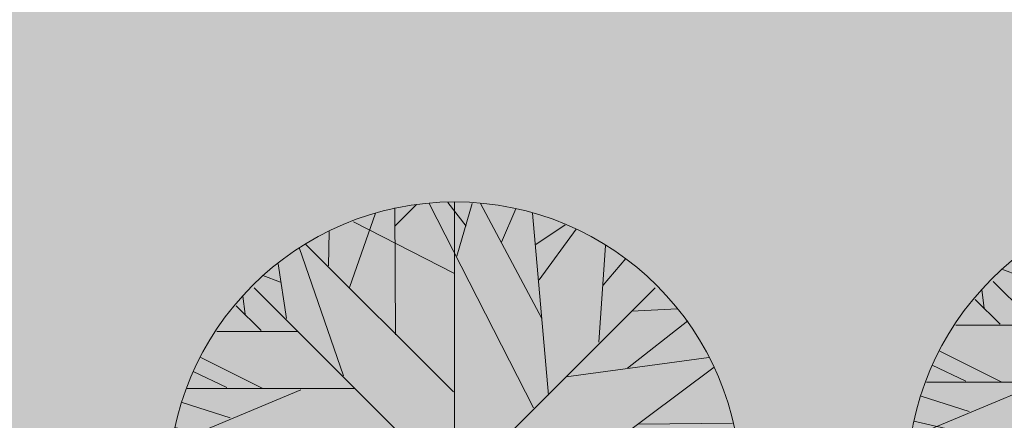
# Model space of a CAD drawing. Units: inches. Extents: x 459864 to 460310, y 324185 to 324787.
# Tile 58 of 112: x 460169 to 460210, y 324222 to 324239. Entities that reach past the tile are written whole.
import ezdxf

# ---------------------------------------------------------------- set-up
doc = ezdxf.new("R2010")
doc.units = ezdxf.units.IN
doc.layers.add('L-PLNT', color=3, linetype='Continuous', lineweight=13)
doc.layers.add('L-SITE-PATT', color=252, linetype='Continuous', lineweight=13)

# ---------------------------------------------------------------- blocks, each defined once
blk = doc.blocks.new('Tree - deciduous plan')
for p, q in [((2.426, 54.9406), (-1.4472, 59.9056)), ((0, 59.9996), (0, -60)), ((-12.5388, 54.9406), (-7.9613, 59.4546)), ((-12.3627, 32.1443), (-12.5388, 58.7776)), ((-5.3205, 59.6806), (16.5105, 16.7963)), ((0.4894, 48.6208), (3.6584, 59.6806)), ((18.2711, 35.5298), (5.419, 59.6806)), ((9.8203, 51.5549), (12.8133, 58.5516)), ((-22.0458, 42.0753), (-16.5881, 57.6486)), ((-21.1656, 55.8436), (-0.0388, 45.0094)), ((19.6795, 19.5047), (16.3344, 57.6486)), ((-26.4472, 46.5894), (-26.2712, 53.8116)), ((17.0387, 51.1035), (23.2006, 55.1666)), ((17.7429, 43.6552), (25.4894, 54.2636)), ((-32.6092, 50.4264), (-23.2782, 23.5674)), ((-31.2008, 51.1035), (-0.2149, 20.1818)), ((31.6513, 50.8778), (30.2429, 30.5643)), ((31.1232, 42.5267), (35.8767, 48.1693)), ((-37.0107, 47.0408), (-35.25, 35.5298)), ((-40.1797, 44.558), (-36.4825, 43.2038)), ((42, 42), (-42, -42)), ((42, -42), (-42, 42)), ((-43.8768, 36.4326), (-44.405, 40.2696)), ((-45.8134, 38.2383), (-40.5318, 33.0471)), ((37.1091, 37.1098), (46.6161, 37.5612)), ((36.2288, 25.1474), (48.9049, 35.0784)), ((-49.8627, 32.8214), (-32.7853, 32.8214)), ((-53.2078, 27.4044), (-40.1797, 20.859)), ((23.3767, 23.3417), (53.3063, 27.4044)), ((54.3626, 25.3731), (20.9119, 0.3198)), ((-54.7923, 24.4702), (-47.75, 21.0847)), ((-56.0247, 20.859), (-20.8134, 20.859)), ((-32.2571, 20.6333), (-59.1937, 9.348)), ((-57.081, 17.9248), (-47.0458, 14.7649)), ((-58.6656, 12.7336), (-35.9543, 7.5424)), ((38.5175, 13.4107), (58.2359, 13.6364)), ((-59.7219, 2.8025), (-12.0106, 12.0565)), ((29.3626, -6.6771), (59.4682, 7.091)), ((-54.6162, -24.7335), (-20.2853, 0.0941)), ((-60, 0), (60, 0)), ((-45.2853, -0.1316), (-59.0177, -10.0627)), ((9.2922, -9.1598), (59.6443, -2.8401)), ((-59.7219, -4.8714), (-54.2641, -6.6771)), ((-10.074, -10.0627), (-2.5036, -59.7178)), ((26.3697, -18.4138), (58.9401, -9.8369)), ((-58.4895, -12.3197), (-36.4825, -11.6426)), ((-14.8275, -15.0282), (-14.6515, -57.6865)), ((-57.081, -18.4138), (-45.2853, -17.9624)), ((-52.6797, -18.188), (-55.4966, -22.0251)), ((-53.2078, -27.442), (-16.7641, -16.6081)), ((18.7992, -18.6394), (57.3556, -17.2853)), ((38.1654, -18.188), (52.426, -29.0219)), ((-47.2219, -19.3166), (-50.2148, -26.3135)), ((-19.9331, -20.2194), (-28.5599, -52.721)), ((-0.0388, -19.0909), (25.8415, -53.8495)), ((18.6232, -18.6394), (26.7218, -53.3981)), ((-35.9543, -22.4765), (-44.0529, -40.5329)), ((45.9119, -24.0564), (55.595, -22.2508)), ((-38.9472, -29.0219), (-51.4472, -30.6018)), ((-46.5177, -30.1504), (-49.5106, -33.536)), ((30.419, -30.1504), (32.3556, -50.0125)), ((-32.4331, -32.4075), (-48.1021, -35.5674)), ((-14.6515, -32.1818), (-3.912, -59.4922)), ((31.4753, -31.279), (49.6091, -33.3103)), ((41.5105, -32.6332), (46.088, -38.0501)), ((-43.7008, -34.6645), (-46.6937, -37.373)), ((-14.6515, -36.2445), (-27.6797, -52.9467)), ((-6.2008, -36.2445), (17.919, -57.0094)), ((22.8485, -36.4702), (35.3485, -48.4326)), ((-24.6867, -37.8244), (-38.7712, -45.7241)), ((-26.2712, -43.9185), (-34.7219, -48.6583)), ((24.7852, -44.8213), (23.0246, -54.978)), ((-14.6515, -47.3041), (-25.0388, -54.3009)), ((-21.5177, -45.4984), (-19.9331, -56.1065)), ((5.9471, -46.6269), (10.5246, -58.5893)), ((-8.4895, -47.5298), (-11.4825, -58.5893)), ((-6.3768, -52.721), (-9.3698, -58.815)), ((8.4119, -53.1724), (3.8344, -59.4922))]:
    blk.add_line(p, q)
blk.add_circle((0, 0), 60)

msp = doc.modelspace()

# ---------------------------------------------------------------- hatches: boundary and pattern name
at = {"layer": 'L-SITE-PATT'}
h = msp.add_hatch(dxfattribs=at)
h.set_pattern_fill('DOTS', color=256)
h.paths.add_polyline_path([(460269.804, 324283.483), (460247.115, 324283.483), (460121.929, 324283.483), (460121.929, 324252.473), (460117.429, 324252.473), (460110.124, 324252.473), (460110.124, 324243.287), (460080.83, 324243.287), (460080.83, 324252.473), (460061.115, 324252.473), (460061.115, 324251.882), (460077.909, 324251.882), (460077.909, 324199.483), (460080.83, 324199.483), (460080.83, 324207.553), (460110.124, 324207.553), (460110.124, 324199.483), (460110.813, 324199.483), (460262.115, 324199.483), (460269.804, 324199.483)], flags=17)
edge = h.paths.add_edge_path(flags=0)
edge.add_ellipse((460222.59, 324263.813), major_axis=(-8.485, 8.485), ratio=1, start_angle=405, end_angle=495, ccw=False)
edge.add_line((460214.821, 324254.66), (460214.832, 324254.666))
edge.add_ellipse((460222.59, 324263.813), major_axis=(-8.485, 8.485), ratio=1, start_angle=405, end_angle=495, ccw=False)
edge.add_line((460210.759, 324261.781), (460210.768, 324261.787))
edge.add_ellipse((460222.59, 324263.813), major_axis=(-8.485, 8.485), ratio=1, start_angle=405, end_angle=495, ccw=False)
edge.add_ellipse((460222.59, 324263.813), major_axis=(-8.485, 8.485), ratio=1, start_angle=392.754, end_angle=405, ccw=False)
edge.add_ellipse((460222.59, 324263.813), major_axis=(-8.485, 8.485), ratio=1, start_angle=380.9347, end_angle=392.754, ccw=False)
edge.add_line((460211.337, 324267.985), (460211.34, 324267.985))
edge.add_ellipse((460222.59, 324263.813), major_axis=(-8.485, 8.485), ratio=1, start_angle=380.9347, end_angle=392.754, ccw=False)
edge.add_ellipse((460222.59, 324263.813), major_axis=(-8.485, 8.485), ratio=1, start_angle=347.9015, end_angle=380.9347, ccw=False)
edge.add_ellipse((460222.59, 324263.813), major_axis=(-8.485, 8.485), ratio=1, start_angle=327.0619, end_angle=347.9015, ccw=False)
edge.add_ellipse((460222.59, 324263.813), major_axis=(-8.485, 8.485), ratio=1, start_angle=278.3246, end_angle=327.0619, ccw=False)
edge.add_line((460225.158, 324275.536), (460225.158, 324275.535))
edge.add_ellipse((460222.59, 324263.813), major_axis=(-8.485, 8.485), ratio=1, start_angle=278.3246, end_angle=327.0619, ccw=False)
edge.add_ellipse((460222.59, 324263.813), major_axis=(-8.485, 8.485), ratio=1, start_angle=260.6436, end_angle=278.3246, ccw=False)
edge.add_ellipse((460222.59, 324263.813), major_axis=(-8.485, 8.485), ratio=1, start_angle=225, end_angle=260.6436, ccw=False)
edge.add_line((460234.509, 324265.243), (460234.501, 324265.239))
edge.add_ellipse((460222.59, 324263.813), major_axis=(-8.485, 8.485), ratio=1, start_angle=225, end_angle=260.6436, ccw=False)
edge.add_ellipse((460222.59, 324263.813), major_axis=(-8.485, 8.485), ratio=1, start_angle=495, end_angle=585, ccw=False)
edge.add_line((460234.437, 324261.861), (460234.424, 324261.858))
edge.add_ellipse((460222.59, 324263.813), major_axis=(-8.485, 8.485), ratio=1, start_angle=495, end_angle=585, ccw=False)
edge.add_line((460227.95, 324253.067), (460227.946, 324253.083))
edge.add_ellipse((460222.59, 324263.813), major_axis=(-8.485, 8.485), ratio=1, start_angle=495, end_angle=585, ccw=False)
edge.add_line((460226.223, 324252.369), (460226.211, 324252.38))
edge.add_ellipse((460222.59, 324263.813), major_axis=(-8.485, 8.485), ratio=1, start_angle=495, end_angle=585, ccw=False)
h.paths.add_polyline_path([(460219.651, 324254.347), (460218.461, 324253.545), (460218.275, 324254.789), (460219.642, 324256.542), (460219.625, 324260.848), (460216.11, 324257.333), (460214.35, 324256.978), (460215.416, 324259.356), (460212.524, 324258.496), (460213.137, 324259.93), (460218.507, 324263.813), (460222.59, 324263.813), (460222.59, 324267.807), (460218.176, 324272.212), (460219.026, 324274.639), (460222.59, 324272.811), (460222.59, 324275.423), (460223.057, 324274.825), (460222.675, 324273.492), (460225.912, 324267.135), (460219.625, 324260.848)], flags=0)
edge = h.paths.add_edge_path(flags=0)
edge.add_ellipse((460194.576, 324264.046), major_axis=(-8.485, 8.485), ratio=1, start_angle=495, end_angle=585, ccw=False)
edge.add_line((460199.936, 324253.3), (460199.932, 324253.316))
edge.add_ellipse((460194.576, 324264.046), major_axis=(-8.485, 8.485), ratio=1, start_angle=495, end_angle=585, ccw=False)
edge.add_line((460198.208, 324252.603), (460198.196, 324252.613))
edge.add_ellipse((460194.576, 324264.046), major_axis=(-8.485, 8.485), ratio=1, start_angle=495, end_angle=585, ccw=False)
edge.add_ellipse((460194.576, 324264.046), major_axis=(-8.485, 8.485), ratio=1, start_angle=405, end_angle=495, ccw=False)
edge.add_line((460186.806, 324254.893), (460186.817, 324254.899))
edge.add_ellipse((460194.576, 324264.046), major_axis=(-8.485, 8.485), ratio=1, start_angle=405, end_angle=495, ccw=False)
edge.add_line((460182.744, 324262.014), (460182.753, 324262.02))
edge.add_ellipse((460194.576, 324264.046), major_axis=(-8.485, 8.485), ratio=1, start_angle=405, end_angle=495, ccw=False)
edge.add_ellipse((460194.576, 324264.046), major_axis=(-8.485, 8.485), ratio=1, start_angle=392.754, end_angle=405, ccw=False)
edge.add_ellipse((460194.576, 324264.046), major_axis=(-8.485, 8.485), ratio=1, start_angle=380.9347, end_angle=392.754, ccw=False)
edge.add_line((460183.323, 324268.218), (460183.326, 324268.218))
edge.add_ellipse((460194.576, 324264.046), major_axis=(-8.485, 8.485), ratio=1, start_angle=380.9347, end_angle=392.754, ccw=False)
edge.add_ellipse((460194.576, 324264.046), major_axis=(-8.485, 8.485), ratio=1, start_angle=347.9015, end_angle=380.9347, ccw=False)
edge.add_ellipse((460194.576, 324264.046), major_axis=(-8.485, 8.485), ratio=1, start_angle=327.0619, end_angle=347.9015, ccw=False)
edge.add_ellipse((460194.576, 324264.046), major_axis=(-8.485, 8.485), ratio=1, start_angle=278.3246, end_angle=327.0619, ccw=False)
edge.add_line((460197.144, 324275.769), (460197.143, 324275.768))
edge.add_ellipse((460194.576, 324264.046), major_axis=(-8.485, 8.485), ratio=1, start_angle=278.3246, end_angle=327.0619, ccw=False)
edge.add_ellipse((460194.576, 324264.046), major_axis=(-8.485, 8.485), ratio=1, start_angle=260.6436, end_angle=278.3246, ccw=False)
edge.add_ellipse((460194.576, 324264.046), major_axis=(-8.485, 8.485), ratio=1, start_angle=225, end_angle=260.6436, ccw=False)
edge.add_line((460206.494, 324265.476), (460206.487, 324265.473))
edge.add_ellipse((460194.576, 324264.046), major_axis=(-8.485, 8.485), ratio=1, start_angle=225, end_angle=260.6436, ccw=False)
edge.add_ellipse((460194.576, 324264.046), major_axis=(-8.485, 8.485), ratio=1, start_angle=495, end_angle=585, ccw=False)
edge.add_line((460206.422, 324262.094), (460206.409, 324262.091))
h.paths.add_polyline_path([(460191.61, 324261.081), (460191.637, 324254.58), (460190.447, 324253.778), (460190.261, 324255.023), (460191.628, 324256.775), (460191.61, 324261.081), (460188.096, 324257.566), (460186.335, 324257.211), (460187.402, 324259.589), (460184.509, 324258.729), (460185.123, 324260.163), (460190.493, 324264.046), (460194.576, 324264.046), (460194.576, 324268.04), (460190.161, 324272.446), (460191.011, 324274.872), (460194.576, 324273.044), (460194.576, 324275.657), (460195.043, 324275.058), (460194.661, 324273.725), (460197.897, 324267.368)], flags=0)
edge = h.paths.add_edge_path(flags=0)
edge.add_ellipse((460252.912, 324263.578), major_axis=(-8.485, 8.485), ratio=1, start_angle=405, end_angle=495, ccw=False)
edge.add_line((460241.081, 324261.545), (460241.089, 324261.551))
edge.add_ellipse((460252.912, 324263.578), major_axis=(-8.485, 8.485), ratio=1, start_angle=405, end_angle=495, ccw=False)
edge.add_ellipse((460252.912, 324263.578), major_axis=(-8.485, 8.485), ratio=1, start_angle=392.754, end_angle=405, ccw=False)
edge.add_ellipse((460252.912, 324263.578), major_axis=(-8.485, 8.485), ratio=1, start_angle=380.9347, end_angle=392.754, ccw=False)
edge.add_line((460241.659, 324267.749), (460241.662, 324267.749))
edge.add_ellipse((460252.912, 324263.578), major_axis=(-8.485, 8.485), ratio=1, start_angle=380.9347, end_angle=392.754, ccw=False)
edge.add_ellipse((460252.912, 324263.578), major_axis=(-8.485, 8.485), ratio=1, start_angle=347.9015, end_angle=380.9347, ccw=False)
edge.add_ellipse((460252.912, 324263.578), major_axis=(-8.485, 8.485), ratio=1, start_angle=327.0619, end_angle=347.9015, ccw=False)
edge.add_ellipse((460252.912, 324263.578), major_axis=(-8.485, 8.485), ratio=1, start_angle=278.3246, end_angle=327.0619, ccw=False)
edge.add_line((460255.48, 324275.3), (460255.479, 324275.299))
edge.add_ellipse((460252.912, 324263.578), major_axis=(-8.485, 8.485), ratio=1, start_angle=278.3246, end_angle=327.0619, ccw=False)
edge.add_ellipse((460252.912, 324263.578), major_axis=(-8.485, 8.485), ratio=1, start_angle=260.6436, end_angle=278.3246, ccw=False)
edge.add_ellipse((460252.912, 324263.578), major_axis=(-8.485, 8.485), ratio=1, start_angle=225, end_angle=260.6436, ccw=False)
edge.add_line((460264.83, 324265.007), (460264.823, 324265.004))
edge.add_ellipse((460252.912, 324263.578), major_axis=(-8.485, 8.485), ratio=1, start_angle=225, end_angle=260.6436, ccw=False)
edge.add_ellipse((460252.912, 324263.578), major_axis=(-8.485, 8.485), ratio=1, start_angle=495, end_angle=585, ccw=False)
edge.add_line((460264.758, 324261.626), (460264.745, 324261.622))
edge.add_ellipse((460252.912, 324263.578), major_axis=(-8.485, 8.485), ratio=1, start_angle=495, end_angle=585, ccw=False)
edge.add_line((460258.272, 324252.832), (460258.268, 324252.848))
edge.add_ellipse((460252.912, 324263.578), major_axis=(-8.485, 8.485), ratio=1, start_angle=495, end_angle=585, ccw=False)
edge.add_line((460256.545, 324252.134), (460256.533, 324252.144))
edge.add_ellipse((460252.912, 324263.578), major_axis=(-8.485, 8.485), ratio=1, start_angle=495, end_angle=585, ccw=False)
edge.add_ellipse((460252.912, 324263.578), major_axis=(-8.485, 8.485), ratio=1, start_angle=405, end_angle=495, ccw=False)
edge.add_line((460245.143, 324254.424), (460245.153, 324254.43))
h.paths.add_polyline_path([(460244.672, 324256.742), (460245.738, 324259.12), (460242.846, 324258.26), (460243.459, 324259.694), (460248.829, 324263.578), (460252.912, 324263.578), (460252.912, 324267.571), (460248.497, 324271.977), (460249.348, 324274.403), (460252.912, 324272.576), (460252.912, 324275.188), (460253.379, 324274.589), (460252.997, 324273.257), (460256.233, 324266.899), (460249.946, 324260.612), (460249.973, 324254.111), (460248.783, 324253.309), (460248.597, 324254.554), (460249.964, 324256.306), (460249.946, 324260.612), (460246.432, 324257.097)], flags=0)
edge = h.paths.add_edge_path(flags=0)
edge.add_ellipse((460167.439, 324262.833), major_axis=(-8.485, 8.485), ratio=1, start_angle=495, end_angle=585, ccw=False)
edge.add_line((460172.799, 324252.087), (460172.795, 324252.103))
edge.add_ellipse((460167.439, 324262.833), major_axis=(-8.485, 8.485), ratio=1, start_angle=495, end_angle=585, ccw=False)
edge.add_line((460171.071, 324251.389), (460171.059, 324251.399))
edge.add_ellipse((460167.439, 324262.833), major_axis=(-8.485, 8.485), ratio=1, start_angle=495, end_angle=585, ccw=False)
edge.add_ellipse((460167.439, 324262.833), major_axis=(-8.485, 8.485), ratio=1, start_angle=405, end_angle=495, ccw=False)
edge.add_line((460159.669, 324253.679), (460159.68, 324253.685))
edge.add_ellipse((460167.439, 324262.833), major_axis=(-8.485, 8.485), ratio=1, start_angle=405, end_angle=495, ccw=False)
edge.add_line((460155.607, 324260.8), (460155.616, 324260.806))
edge.add_ellipse((460167.439, 324262.833), major_axis=(-8.485, 8.485), ratio=1, start_angle=405, end_angle=495, ccw=False)
edge.add_ellipse((460167.439, 324262.833), major_axis=(-8.485, 8.485), ratio=1, start_angle=392.754, end_angle=405, ccw=False)
edge.add_ellipse((460167.439, 324262.833), major_axis=(-8.485, 8.485), ratio=1, start_angle=380.9347, end_angle=392.754, ccw=False)
edge.add_line((460156.185, 324267.005), (460156.189, 324267.005))
edge.add_ellipse((460167.439, 324262.833), major_axis=(-8.485, 8.485), ratio=1, start_angle=380.9347, end_angle=392.754, ccw=False)
edge.add_ellipse((460167.439, 324262.833), major_axis=(-8.485, 8.485), ratio=1, start_angle=347.9015, end_angle=380.9347, ccw=False)
edge.add_ellipse((460167.439, 324262.833), major_axis=(-8.485, 8.485), ratio=1, start_angle=327.0619, end_angle=347.9015, ccw=False)
edge.add_ellipse((460167.439, 324262.833), major_axis=(-8.485, 8.485), ratio=1, start_angle=278.3246, end_angle=327.0619, ccw=False)
edge.add_line((460170.007, 324274.556), (460170.006, 324274.554))
edge.add_ellipse((460167.439, 324262.833), major_axis=(-8.485, 8.485), ratio=1, start_angle=278.3246, end_angle=327.0619, ccw=False)
edge.add_ellipse((460167.439, 324262.833), major_axis=(-8.485, 8.485), ratio=1, start_angle=260.6436, end_angle=278.3246, ccw=False)
edge.add_ellipse((460167.439, 324262.833), major_axis=(-8.485, 8.485), ratio=1, start_angle=225, end_angle=260.6436, ccw=False)
edge.add_line((460179.357, 324264.262), (460179.35, 324264.259))
edge.add_ellipse((460167.439, 324262.833), major_axis=(-8.485, 8.485), ratio=1, start_angle=225, end_angle=260.6436, ccw=False)
edge.add_ellipse((460167.439, 324262.833), major_axis=(-8.485, 8.485), ratio=1, start_angle=495, end_angle=585, ccw=False)
edge.add_line((460179.285, 324260.881), (460179.272, 324260.877))
h.paths.add_polyline_path([(460164.473, 324259.867), (460164.5, 324253.366), (460163.31, 324252.565), (460163.124, 324253.809), (460164.491, 324255.561), (460164.473, 324259.867), (460160.958, 324256.353), (460159.198, 324255.998), (460160.265, 324258.375), (460157.372, 324257.515), (460157.986, 324258.949), (460163.356, 324262.833), (460167.439, 324262.833), (460167.439, 324266.826), (460163.024, 324271.232), (460163.874, 324273.659), (460167.439, 324271.831), (460167.439, 324274.443), (460167.905, 324273.844), (460167.524, 324272.512), (460170.76, 324266.154)], flags=0)
edge = h.paths.add_edge_path(flags=0)
edge.add_ellipse((460140.758, 324262.37), major_axis=(-8.485, 8.485), ratio=1, start_angle=495, end_angle=585, ccw=False)
edge.add_line((460146.118, 324251.624), (460146.114, 324251.639))
edge.add_ellipse((460140.758, 324262.37), major_axis=(-8.485, 8.485), ratio=1, start_angle=495, end_angle=585, ccw=False)
edge.add_line((460144.391, 324250.926), (460144.379, 324250.936))
edge.add_ellipse((460140.758, 324262.37), major_axis=(-8.485, 8.485), ratio=1, start_angle=495, end_angle=585, ccw=False)
edge.add_ellipse((460140.758, 324262.37), major_axis=(-8.485, 8.485), ratio=1, start_angle=405, end_angle=495, ccw=False)
edge.add_line((460132.989, 324253.216), (460132.999, 324253.222))
edge.add_ellipse((460140.758, 324262.37), major_axis=(-8.485, 8.485), ratio=1, start_angle=405, end_angle=495, ccw=False)
edge.add_line((460128.927, 324260.337), (460128.935, 324260.343))
edge.add_ellipse((460140.758, 324262.37), major_axis=(-8.485, 8.485), ratio=1, start_angle=405, end_angle=495, ccw=False)
edge.add_ellipse((460140.758, 324262.37), major_axis=(-8.485, 8.485), ratio=1, start_angle=392.754, end_angle=405, ccw=False)
edge.add_ellipse((460140.758, 324262.37), major_axis=(-8.485, 8.485), ratio=1, start_angle=380.9347, end_angle=392.754, ccw=False)
edge.add_line((460129.505, 324266.541), (460129.508, 324266.541))
edge.add_ellipse((460140.758, 324262.37), major_axis=(-8.485, 8.485), ratio=1, start_angle=380.9347, end_angle=392.754, ccw=False)
edge.add_ellipse((460140.758, 324262.37), major_axis=(-8.485, 8.485), ratio=1, start_angle=347.9015, end_angle=380.9347, ccw=False)
edge.add_ellipse((460140.758, 324262.37), major_axis=(-8.485, 8.485), ratio=1, start_angle=327.0619, end_angle=347.9015, ccw=False)
edge.add_ellipse((460140.758, 324262.37), major_axis=(-8.485, 8.485), ratio=1, start_angle=278.3246, end_angle=327.0619, ccw=False)
edge.add_line((460143.326, 324274.092), (460143.325, 324274.091))
edge.add_ellipse((460140.758, 324262.37), major_axis=(-8.485, 8.485), ratio=1, start_angle=278.3246, end_angle=327.0619, ccw=False)
edge.add_ellipse((460140.758, 324262.37), major_axis=(-8.485, 8.485), ratio=1, start_angle=260.6436, end_angle=278.3246, ccw=False)
edge.add_ellipse((460140.758, 324262.37), major_axis=(-8.485, 8.485), ratio=1, start_angle=225, end_angle=260.6436, ccw=False)
edge.add_line((460152.677, 324263.799), (460152.669, 324263.796))
edge.add_ellipse((460140.758, 324262.37), major_axis=(-8.485, 8.485), ratio=1, start_angle=225, end_angle=260.6436, ccw=False)
edge.add_ellipse((460140.758, 324262.37), major_axis=(-8.485, 8.485), ratio=1, start_angle=495, end_angle=585, ccw=False)
edge.add_line((460152.604, 324260.418), (460152.592, 324260.414))
h.paths.add_polyline_path([(460137.792, 324259.404), (460137.819, 324252.903), (460136.629, 324252.101), (460136.443, 324253.346), (460137.81, 324255.098), (460137.792, 324259.404), (460134.278, 324255.889), (460132.518, 324255.534), (460133.584, 324257.912), (460130.692, 324257.052), (460131.305, 324258.486), (460136.675, 324262.37), (460140.758, 324262.37), (460140.758, 324266.363), (460136.343, 324270.769), (460137.194, 324273.195), (460140.758, 324271.367), (460140.758, 324273.98), (460141.225, 324273.381), (460140.843, 324272.049), (460144.079, 324265.691)], flags=0)
h.paths.add_polyline_path([(460110.124, 324227.414), (460080.83, 324227.414), (460080.83, 324235.484), (460110.124, 324235.484)], flags=16)
h.paths.add_polyline_path([(460110.124, 324220.797), (460110.124, 324212.727), (460080.83, 324212.727), (460080.83, 324220.797)], flags=16)
h.paths.add_polyline_path([(460269.804, 324283.483), (460247.115, 324283.483), (460121.929, 324283.483), (460121.929, 324252.473), (460117.429, 324252.473), (460110.124, 324252.473), (460110.124, 324243.287), (460080.83, 324243.287), (460080.83, 324252.473), (460061.115, 324252.473), (460061.115, 324251.882), (460077.909, 324251.882), (460077.909, 324199.483), (460080.83, 324199.483), (460080.83, 324207.553), (460110.124, 324207.553), (460110.124, 324199.483), (460262.115, 324199.483), (460269.804, 324199.483)], flags=17)
h.paths.add_polyline_path([(460219.651, 324254.347), (460218.461, 324253.545), (460218.275, 324254.789), (460219.642, 324256.542), (460219.625, 324260.848), (460216.11, 324257.333), (460214.35, 324256.978), (460215.416, 324259.356), (460212.524, 324258.496), (460213.137, 324259.93), (460218.507, 324263.813), (460222.59, 324263.813), (460220.18, 324266.223), (460215.461, 324265.308), (460211.835, 324266.137), (460216.247, 324267.985), (460218.418, 324267.985), (460222.59, 324263.813), (460222.59, 324267.807), (460218.176, 324272.212), (460219.026, 324274.639), (460222.59, 324272.811), (460222.59, 324275.423), (460223.057, 324274.825), (460222.675, 324273.492), (460225.912, 324267.135), (460222.59, 324263.813), (460231.383, 324263.813), (460228.485, 324262.488), (460224.425, 324261.978), (460228.68, 324257.724), (460228.966, 324254.791), (460227.142, 324256.537), (460227.542, 324254.819), (460227.333, 324253.614), (460222.59, 324259.985), (460222.59, 324255.497), (460221.377, 324256.541), (460220.576, 324261.799), (460219.625, 324260.848)], flags=0)
h.paths.add_polyline_path([(460199.127, 324256.77), (460199.528, 324255.052), (460199.319, 324253.848), (460194.576, 324260.218), (460194.576, 324255.73), (460193.363, 324256.774), (460192.561, 324262.032), (460191.61, 324261.081), (460191.637, 324254.58), (460190.447, 324253.778), (460190.261, 324255.023), (460191.628, 324256.775), (460191.61, 324261.081), (460188.096, 324257.566), (460186.335, 324257.211), (460187.402, 324259.589), (460184.509, 324258.729), (460185.123, 324260.163), (460190.493, 324264.046), (460194.576, 324264.046), (460192.166, 324266.456), (460187.446, 324265.541), (460183.82, 324266.37), (460188.232, 324268.218), (460190.404, 324268.218), (460194.576, 324264.046), (460194.576, 324268.04), (460190.161, 324272.446), (460191.011, 324274.872), (460194.576, 324273.044), (460194.576, 324275.657), (460195.043, 324275.058), (460194.661, 324273.725), (460197.897, 324267.368), (460194.576, 324264.046), (460203.368, 324264.046), (460200.47, 324262.721), (460196.411, 324262.212), (460200.665, 324257.957), (460200.951, 324255.024)], flags=0)
h.paths.add_polyline_path([(460244.672, 324256.742), (460245.738, 324259.12), (460242.846, 324258.26), (460243.459, 324259.694), (460248.829, 324263.578), (460252.912, 324263.578), (460250.502, 324265.987), (460245.783, 324265.072), (460242.156, 324265.901), (460246.568, 324267.749), (460248.74, 324267.749), (460252.912, 324263.578), (460252.912, 324267.571), (460248.497, 324271.977), (460249.348, 324274.403), (460252.912, 324272.576), (460252.912, 324275.188), (460253.379, 324274.589), (460252.997, 324273.257), (460256.233, 324266.899), (460252.912, 324263.578), (460261.705, 324263.578), (460258.806, 324262.252), (460254.747, 324261.743), (460259.002, 324257.488), (460259.288, 324254.555), (460257.463, 324256.301), (460257.864, 324254.583), (460257.655, 324253.379), (460252.912, 324259.749), (460252.912, 324255.261), (460251.699, 324256.305), (460250.897, 324261.563), (460249.946, 324260.612), (460249.973, 324254.111), (460248.783, 324253.309), (460248.597, 324254.554), (460249.964, 324256.306), (460249.946, 324260.612), (460246.432, 324257.097)], flags=0)
h.paths.add_polyline_path([(460173.528, 324256.743), (460173.814, 324253.811), (460171.99, 324255.556), (460172.39, 324253.838), (460172.182, 324252.634), (460167.439, 324259.004), (460167.439, 324254.516), (460166.226, 324255.56), (460165.424, 324260.818), (460164.473, 324259.867), (460164.5, 324253.366), (460163.31, 324252.565), (460163.124, 324253.809), (460164.491, 324255.561), (460164.473, 324259.867), (460160.958, 324256.353), (460159.198, 324255.998), (460160.265, 324258.375), (460157.372, 324257.515), (460157.986, 324258.949), (460163.356, 324262.833), (460167.439, 324262.833), (460165.029, 324265.243), (460160.309, 324264.327), (460156.683, 324265.156), (460161.095, 324267.005), (460163.267, 324267.005), (460167.439, 324262.833), (460167.439, 324266.826), (460163.024, 324271.232), (460163.874, 324273.659), (460167.439, 324271.831), (460167.439, 324274.443), (460167.905, 324273.844), (460167.524, 324272.512), (460170.76, 324266.154), (460167.439, 324262.833), (460176.231, 324262.833), (460173.333, 324261.507), (460169.274, 324260.998)], flags=0)
h.paths.add_polyline_path([(460146.848, 324256.28), (460147.134, 324253.347), (460145.31, 324255.093), (460145.71, 324253.375), (460145.501, 324252.171), (460140.758, 324258.541), (460140.758, 324254.053), (460139.545, 324255.097), (460138.744, 324260.355), (460137.792, 324259.404), (460137.819, 324252.903), (460136.629, 324252.101), (460136.443, 324253.346), (460137.81, 324255.098), (460137.792, 324259.404), (460134.278, 324255.889), (460132.518, 324255.534), (460133.584, 324257.912), (460130.692, 324257.052), (460131.305, 324258.486), (460136.675, 324262.37), (460140.758, 324262.37), (460138.348, 324264.779), (460133.629, 324263.864), (460130.002, 324264.693), (460134.414, 324266.541), (460136.586, 324266.541), (460140.758, 324262.37), (460140.758, 324266.363), (460136.343, 324270.769), (460137.194, 324273.195), (460140.758, 324271.367), (460140.758, 324273.98), (460141.225, 324273.381), (460140.843, 324272.049), (460144.079, 324265.691), (460140.758, 324262.37), (460149.551, 324262.37), (460146.653, 324261.044), (460142.593, 324260.535)], flags=0)
edge = h.paths.add_edge_path()
edge.add_line((460269.804, 324272.549), (460260.881, 324272.549))
edge.add_ellipse((460252.912, 324263.578), major_axis=(-8.485, 8.485), ratio=1, start_angle=260.6436, end_angle=273.3846, ccw=False)
edge.add_line((460262.283, 324271.092), (460262.261, 324271.091))
edge.add_ellipse((460252.912, 324263.578), major_axis=(-8.485, 8.485), ratio=1, start_angle=260.6436, end_angle=273.3846, ccw=False)
edge.add_ellipse((460252.912, 324263.578), major_axis=(-8.485, 8.485), ratio=1, start_angle=225, end_angle=260.6436, ccw=False)
edge.add_line((460263.609, 324269.063), (460263.572, 324269.058))
edge.add_ellipse((460252.912, 324263.578), major_axis=(-8.485, 8.485), ratio=1, start_angle=225, end_angle=260.6436, ccw=False)
edge.add_line((460264.615, 324266.306), (460264.585, 324266.305))
edge.add_ellipse((460252.912, 324263.578), major_axis=(-8.485, 8.485), ratio=1, start_angle=225, end_angle=260.6436, ccw=False)
edge.add_line((460264.83, 324265.007), (460264.823, 324265.004))
edge.add_ellipse((460252.912, 324263.578), major_axis=(-8.485, 8.485), ratio=1, start_angle=225, end_angle=260.6436, ccw=False)
edge.add_ellipse((460252.912, 324263.578), major_axis=(-8.485, 8.485), ratio=1, start_angle=495, end_angle=585, ccw=False)
edge.add_line((460264.758, 324261.626), (460264.745, 324261.622))
edge.add_ellipse((460252.912, 324263.578), major_axis=(-8.485, 8.485), ratio=1, start_angle=495, end_angle=585, ccw=False)
edge.add_line((460263.442, 324257.739), (460263.389, 324257.779))
edge.add_ellipse((460252.912, 324263.578), major_axis=(-8.485, 8.485), ratio=1, start_angle=495, end_angle=585, ccw=False)
edge.add_line((460258.128, 324252.744), (460258.102, 324252.779))
edge.add_ellipse((460252.912, 324263.578), major_axis=(-8.485, 8.485), ratio=1, start_angle=495, end_angle=585, ccw=False)
edge.add_line((460256.545, 324252.134), (460256.533, 324252.144))
edge.add_ellipse((460252.912, 324263.578), major_axis=(-8.485, 8.485), ratio=1, start_angle=495, end_angle=585, ccw=False)
edge.add_ellipse((460252.912, 324263.578), major_axis=(-8.485, 8.485), ratio=1, start_angle=405, end_angle=495, ccw=False)
edge.add_line((460250.594, 324251.78), (460250.605, 324251.82))
edge.add_ellipse((460252.912, 324263.578), major_axis=(-8.485, 8.485), ratio=1, start_angle=405, end_angle=495, ccw=False)
edge.add_line((460245.143, 324254.424), (460245.153, 324254.43))
edge.add_ellipse((460252.912, 324263.578), major_axis=(-8.485, 8.485), ratio=1, start_angle=405, end_angle=495, ccw=False)
edge.add_line((460243.525, 324256.059), (460243.56, 324256.091))
edge.add_ellipse((460252.912, 324263.578), major_axis=(-8.485, 8.485), ratio=1, start_angle=405, end_angle=495, ccw=False)
edge.add_line((460241.44, 324259.893), (460241.522, 324259.896))
edge.add_ellipse((460252.912, 324263.578), major_axis=(-8.485, 8.485), ratio=1, start_angle=405, end_angle=495, ccw=False)
edge.add_line((460241.081, 324261.545), (460241.089, 324261.551))
edge.add_ellipse((460252.912, 324263.578), major_axis=(-8.485, 8.485), ratio=1, start_angle=405, end_angle=495, ccw=False)
edge.add_ellipse((460252.912, 324263.578), major_axis=(-8.485, 8.485), ratio=1, start_angle=392.754, end_angle=405, ccw=False)
edge.add_line((460241.05, 324265.438), (460241.063, 324265.443))
edge.add_ellipse((460252.912, 324263.578), major_axis=(-8.485, 8.485), ratio=1, start_angle=392.754, end_angle=405, ccw=False)
edge.add_ellipse((460252.912, 324263.578), major_axis=(-8.485, 8.485), ratio=1, start_angle=380.9347, end_angle=392.754, ccw=False)
edge.add_line((460241.452, 324267.176), (460241.469, 324267.171))
edge.add_ellipse((460252.912, 324263.578), major_axis=(-8.485, 8.485), ratio=1, start_angle=380.9347, end_angle=392.754, ccw=False)
edge.add_line((460241.659, 324267.749), (460241.662, 324267.749))
edge.add_ellipse((460252.912, 324263.578), major_axis=(-8.485, 8.485), ratio=1, start_angle=380.9347, end_angle=392.754, ccw=False)
edge.add_ellipse((460252.912, 324263.578), major_axis=(-8.485, 8.485), ratio=1, start_angle=356.6154, end_angle=380.9347, ccw=False)
edge.add_line((460244.88, 324272.488), (460244.713, 324272.549))
edge.add_line((460244.713, 324272.549), (460230.817, 324272.549))
edge.add_ellipse((460222.59, 324263.813), major_axis=(-8.485, 8.485), ratio=1, start_angle=260.6436, end_angle=271.7178, ccw=False)
edge.add_ellipse((460222.59, 324263.813), major_axis=(-8.485, 8.485), ratio=1, start_angle=225, end_angle=260.6436, ccw=False)
edge.add_line((460233.287, 324269.299), (460233.25, 324269.294))
edge.add_ellipse((460222.59, 324263.813), major_axis=(-8.485, 8.485), ratio=1, start_angle=225, end_angle=260.6436, ccw=False)
edge.add_line((460234.294, 324266.541), (460234.264, 324266.541))
edge.add_ellipse((460222.59, 324263.813), major_axis=(-8.485, 8.485), ratio=1, start_angle=225, end_angle=260.6436, ccw=False)
edge.add_line((460234.509, 324265.243), (460234.501, 324265.239))
edge.add_ellipse((460222.59, 324263.813), major_axis=(-8.485, 8.485), ratio=1, start_angle=225, end_angle=260.6436, ccw=False)
edge.add_ellipse((460222.59, 324263.813), major_axis=(-8.485, 8.485), ratio=1, start_angle=495, end_angle=585, ccw=False)
edge.add_line((460234.437, 324261.861), (460234.424, 324261.858))
edge.add_ellipse((460222.59, 324263.813), major_axis=(-8.485, 8.485), ratio=1, start_angle=495, end_angle=585, ccw=False)
edge.add_line((460233.121, 324257.975), (460233.068, 324258.015))
edge.add_ellipse((460222.59, 324263.813), major_axis=(-8.485, 8.485), ratio=1, start_angle=495, end_angle=585, ccw=False)
edge.add_line((460227.806, 324252.979), (460227.78, 324253.014))
edge.add_ellipse((460222.59, 324263.813), major_axis=(-8.485, 8.485), ratio=1, start_angle=495, end_angle=585, ccw=False)
edge.add_line((460226.223, 324252.369), (460226.211, 324252.38))
edge.add_ellipse((460222.59, 324263.813), major_axis=(-8.485, 8.485), ratio=1, start_angle=495, end_angle=585, ccw=False)
edge.add_ellipse((460222.59, 324263.813), major_axis=(-8.485, 8.485), ratio=1, start_angle=405, end_angle=495, ccw=False)
edge.add_line((460220.272, 324252.016), (460220.283, 324252.055))
edge.add_ellipse((460222.59, 324263.813), major_axis=(-8.485, 8.485), ratio=1, start_angle=405, end_angle=495, ccw=False)
edge.add_line((460214.821, 324254.66), (460214.832, 324254.666))
edge.add_ellipse((460222.59, 324263.813), major_axis=(-8.485, 8.485), ratio=1, start_angle=405, end_angle=495, ccw=False)
edge.add_line((460213.203, 324256.295), (460213.239, 324256.327))
edge.add_ellipse((460222.59, 324263.813), major_axis=(-8.485, 8.485), ratio=1, start_angle=405, end_angle=495, ccw=False)
edge.add_line((460211.118, 324260.128), (460211.201, 324260.131))
edge.add_ellipse((460222.59, 324263.813), major_axis=(-8.485, 8.485), ratio=1, start_angle=405, end_angle=495, ccw=False)
edge.add_line((460210.759, 324261.781), (460210.768, 324261.787))
edge.add_ellipse((460222.59, 324263.813), major_axis=(-8.485, 8.485), ratio=1, start_angle=405, end_angle=495, ccw=False)
edge.add_ellipse((460222.59, 324263.813), major_axis=(-8.485, 8.485), ratio=1, start_angle=392.754, end_angle=405, ccw=False)
edge.add_line((460210.729, 324265.673), (460210.741, 324265.678))
edge.add_ellipse((460222.59, 324263.813), major_axis=(-8.485, 8.485), ratio=1, start_angle=392.754, end_angle=405, ccw=False)
edge.add_ellipse((460222.59, 324263.813), major_axis=(-8.485, 8.485), ratio=1, start_angle=380.9347, end_angle=392.754, ccw=False)
edge.add_line((460211.13, 324267.412), (460211.147, 324267.407))
edge.add_ellipse((460222.59, 324263.813), major_axis=(-8.485, 8.485), ratio=1, start_angle=380.9347, end_angle=392.754, ccw=False)
edge.add_line((460211.337, 324267.985), (460211.34, 324267.985))
edge.add_ellipse((460222.59, 324263.813), major_axis=(-8.485, 8.485), ratio=1, start_angle=380.9347, end_angle=392.754, ccw=False)
edge.add_ellipse((460222.59, 324263.813), major_axis=(-8.485, 8.485), ratio=1, start_angle=358.2822, end_angle=380.9347, ccw=False)
edge.add_line((460213.705, 324271.902), (460213.709, 324271.869))
edge.add_ellipse((460222.59, 324263.813), major_axis=(-8.485, 8.485), ratio=1, start_angle=358.2822, end_angle=380.9347, ccw=False)
edge.add_line((460214.363, 324272.549), (460203.078, 324272.549))
edge.add_line((460203.078, 324272.549), (460203.06, 324272.531))
edge.add_ellipse((460194.576, 324264.046), major_axis=(-8.485, 8.485), ratio=1, start_angle=260.6436, end_angle=270.1168, ccw=False)
edge.add_line((460203.957, 324271.561), (460203.921, 324271.56))
edge.add_ellipse((460194.576, 324264.046), major_axis=(-8.485, 8.485), ratio=1, start_angle=260.6436, end_angle=270.1168, ccw=False)
edge.add_ellipse((460194.576, 324264.046), major_axis=(-8.485, 8.485), ratio=1, start_angle=225, end_angle=260.6436, ccw=False)
edge.add_line((460205.272, 324269.532), (460205.235, 324269.527))
edge.add_ellipse((460194.576, 324264.046), major_axis=(-8.485, 8.485), ratio=1, start_angle=225, end_angle=260.6436, ccw=False)
edge.add_line((460206.279, 324266.774), (460206.249, 324266.774))
edge.add_ellipse((460194.576, 324264.046), major_axis=(-8.485, 8.485), ratio=1, start_angle=225, end_angle=260.6436, ccw=False)
edge.add_line((460206.494, 324265.476), (460206.487, 324265.473))
edge.add_ellipse((460194.576, 324264.046), major_axis=(-8.485, 8.485), ratio=1, start_angle=225, end_angle=260.6436, ccw=False)
edge.add_ellipse((460194.576, 324264.046), major_axis=(-8.485, 8.485), ratio=1, start_angle=495, end_angle=585, ccw=False)
edge.add_line((460206.422, 324262.094), (460206.409, 324262.091))
edge.add_ellipse((460194.576, 324264.046), major_axis=(-8.485, 8.485), ratio=1, start_angle=495, end_angle=585, ccw=False)
edge.add_line((460205.106, 324258.208), (460205.053, 324258.248))
edge.add_ellipse((460194.576, 324264.046), major_axis=(-8.485, 8.485), ratio=1, start_angle=495, end_angle=585, ccw=False)
edge.add_line((460199.792, 324253.212), (460199.766, 324253.248))
edge.add_ellipse((460194.576, 324264.046), major_axis=(-8.485, 8.485), ratio=1, start_angle=495, end_angle=585, ccw=False)
edge.add_line((460198.208, 324252.603), (460198.196, 324252.613))
edge.add_ellipse((460194.576, 324264.046), major_axis=(-8.485, 8.485), ratio=1, start_angle=495, end_angle=585, ccw=False)
edge.add_ellipse((460194.576, 324264.046), major_axis=(-8.485, 8.485), ratio=1, start_angle=405, end_angle=495, ccw=False)
edge.add_line((460192.258, 324252.249), (460192.268, 324252.289))
edge.add_ellipse((460194.576, 324264.046), major_axis=(-8.485, 8.485), ratio=1, start_angle=405, end_angle=495, ccw=False)
edge.add_line((460186.806, 324254.893), (460186.817, 324254.899))
edge.add_ellipse((460194.576, 324264.046), major_axis=(-8.485, 8.485), ratio=1, start_angle=405, end_angle=495, ccw=False)
edge.add_line((460185.188, 324256.528), (460185.224, 324256.56))
edge.add_ellipse((460194.576, 324264.046), major_axis=(-8.485, 8.485), ratio=1, start_angle=405, end_angle=495, ccw=False)
edge.add_line((460183.104, 324260.362), (460183.186, 324260.365))
edge.add_ellipse((460194.576, 324264.046), major_axis=(-8.485, 8.485), ratio=1, start_angle=405, end_angle=495, ccw=False)
edge.add_line((460182.744, 324262.014), (460182.753, 324262.02))
edge.add_ellipse((460194.576, 324264.046), major_axis=(-8.485, 8.485), ratio=1, start_angle=405, end_angle=495, ccw=False)
edge.add_ellipse((460194.576, 324264.046), major_axis=(-8.485, 8.485), ratio=1, start_angle=392.754, end_angle=405, ccw=False)
edge.add_line((460182.714, 324265.906), (460182.726, 324265.912))
edge.add_ellipse((460194.576, 324264.046), major_axis=(-8.485, 8.485), ratio=1, start_angle=392.754, end_angle=405, ccw=False)
edge.add_ellipse((460194.576, 324264.046), major_axis=(-8.485, 8.485), ratio=1, start_angle=380.9347, end_angle=392.754, ccw=False)
edge.add_line((460183.116, 324267.645), (460183.133, 324267.64))
edge.add_ellipse((460194.576, 324264.046), major_axis=(-8.485, 8.485), ratio=1, start_angle=380.9347, end_angle=392.754, ccw=False)
edge.add_line((460183.323, 324268.218), (460183.326, 324268.218))
edge.add_ellipse((460194.576, 324264.046), major_axis=(-8.485, 8.485), ratio=1, start_angle=380.9347, end_angle=392.754, ccw=False)
edge.add_ellipse((460194.576, 324264.046), major_axis=(-8.485, 8.485), ratio=1, start_angle=359.8832, end_angle=380.9347, ccw=False)
edge.add_line((460184.491, 324270.611), (460184.553, 324270.611))
edge.add_ellipse((460194.576, 324264.046), major_axis=(-8.485, 8.485), ratio=1, start_angle=359.8832, end_angle=380.9347, ccw=False)
edge.add_line((460185.346, 324271.76), (460185.379, 324271.728))
edge.add_ellipse((460194.576, 324264.046), major_axis=(-8.485, 8.485), ratio=1, start_angle=359.8832, end_angle=380.9347, ccw=False)
edge.add_line((460185.697, 324272.086), (460185.633, 324272.549))
edge.add_line((460185.633, 324272.549), (460174.683, 324272.549))
edge.add_line((460174.683, 324272.549), (460174.606, 324272.457))
edge.add_ellipse((460167.439, 324262.833), major_axis=(-8.485, 8.485), ratio=1, start_angle=260.6436, end_angle=278.3246, ccw=False)
edge.add_ellipse((460167.439, 324262.833), major_axis=(-8.485, 8.485), ratio=1, start_angle=225, end_angle=260.6436, ccw=False)
edge.add_line((460178.135, 324268.318), (460178.098, 324268.313))
edge.add_ellipse((460167.439, 324262.833), major_axis=(-8.485, 8.485), ratio=1, start_angle=225, end_angle=260.6436, ccw=False)
edge.add_line((460179.142, 324265.561), (460179.112, 324265.56))
edge.add_ellipse((460167.439, 324262.833), major_axis=(-8.485, 8.485), ratio=1, start_angle=225, end_angle=260.6436, ccw=False)
edge.add_line((460179.357, 324264.262), (460179.35, 324264.259))
edge.add_ellipse((460167.439, 324262.833), major_axis=(-8.485, 8.485), ratio=1, start_angle=225, end_angle=260.6436, ccw=False)
edge.add_ellipse((460167.439, 324262.833), major_axis=(-8.485, 8.485), ratio=1, start_angle=495, end_angle=585, ccw=False)
edge.add_line((460179.285, 324260.881), (460179.272, 324260.877))
edge.add_ellipse((460167.439, 324262.833), major_axis=(-8.485, 8.485), ratio=1, start_angle=495, end_angle=585, ccw=False)
edge.add_line((460177.969, 324256.994), (460177.916, 324257.034))
edge.add_ellipse((460167.439, 324262.833), major_axis=(-8.485, 8.485), ratio=1, start_angle=495, end_angle=585, ccw=False)
edge.add_line((460172.655, 324251.999), (460172.629, 324252.034))
edge.add_ellipse((460167.439, 324262.833), major_axis=(-8.485, 8.485), ratio=1, start_angle=495, end_angle=585, ccw=False)
edge.add_line((460171.071, 324251.389), (460171.059, 324251.399))
edge.add_ellipse((460167.439, 324262.833), major_axis=(-8.485, 8.485), ratio=1, start_angle=495, end_angle=585, ccw=False)
edge.add_ellipse((460167.439, 324262.833), major_axis=(-8.485, 8.485), ratio=1, start_angle=405, end_angle=495, ccw=False)
edge.add_line((460165.121, 324251.036), (460165.131, 324251.075))
edge.add_ellipse((460167.439, 324262.833), major_axis=(-8.485, 8.485), ratio=1, start_angle=405, end_angle=495, ccw=False)
edge.add_line((460159.669, 324253.679), (460159.68, 324253.685))
edge.add_ellipse((460167.439, 324262.833), major_axis=(-8.485, 8.485), ratio=1, start_angle=405, end_angle=495, ccw=False)
edge.add_line((460158.051, 324255.314), (460158.087, 324255.347))
edge.add_ellipse((460167.439, 324262.833), major_axis=(-8.485, 8.485), ratio=1, start_angle=405, end_angle=495, ccw=False)
edge.add_line((460155.967, 324259.148), (460156.049, 324259.151))
edge.add_ellipse((460167.439, 324262.833), major_axis=(-8.485, 8.485), ratio=1, start_angle=405, end_angle=495, ccw=False)
edge.add_line((460155.607, 324260.8), (460155.616, 324260.806))
edge.add_ellipse((460167.439, 324262.833), major_axis=(-8.485, 8.485), ratio=1, start_angle=405, end_angle=495, ccw=False)
edge.add_ellipse((460167.439, 324262.833), major_axis=(-8.485, 8.485), ratio=1, start_angle=392.754, end_angle=405, ccw=False)
edge.add_line((460155.577, 324264.693), (460155.589, 324264.698))
edge.add_ellipse((460167.439, 324262.833), major_axis=(-8.485, 8.485), ratio=1, start_angle=392.754, end_angle=405, ccw=False)
edge.add_ellipse((460167.439, 324262.833), major_axis=(-8.485, 8.485), ratio=1, start_angle=380.9347, end_angle=392.754, ccw=False)
edge.add_line((460155.979, 324266.432), (460155.996, 324266.426))
edge.add_ellipse((460167.439, 324262.833), major_axis=(-8.485, 8.485), ratio=1, start_angle=380.9347, end_angle=392.754, ccw=False)
edge.add_line((460156.185, 324267.005), (460156.189, 324267.005))
edge.add_ellipse((460167.439, 324262.833), major_axis=(-8.485, 8.485), ratio=1, start_angle=380.9347, end_angle=392.754, ccw=False)
edge.add_ellipse((460167.439, 324262.833), major_axis=(-8.485, 8.485), ratio=1, start_angle=350.9345, end_angle=380.9347, ccw=False)
edge.add_line((460157.363, 324269.397), (460157.414, 324269.397))
edge.add_ellipse((460167.439, 324262.833), major_axis=(-8.485, 8.485), ratio=1, start_angle=350.9345, end_angle=380.9347, ccw=False)
edge.add_line((460158.221, 324270.535), (460158.236, 324270.519))
edge.add_ellipse((460167.439, 324262.833), major_axis=(-8.485, 8.485), ratio=1, start_angle=350.9345, end_angle=380.9347, ccw=False)
edge.add_line((460159.379, 324271.753), (460159.419, 324271.738))
edge.add_ellipse((460167.439, 324262.833), major_axis=(-8.485, 8.485), ratio=1, start_angle=350.9345, end_angle=380.9347, ccw=False)
edge.add_line((460160.396, 324272.549), (460147.112, 324272.549))
edge.add_ellipse((460140.758, 324262.37), major_axis=(-8.485, 8.485), ratio=1, start_angle=278.3246, end_angle=283.0261, ccw=False)
edge.add_ellipse((460140.758, 324262.37), major_axis=(-8.485, 8.485), ratio=1, start_angle=260.6436, end_angle=278.3246, ccw=False)
edge.add_ellipse((460140.758, 324262.37), major_axis=(-8.485, 8.485), ratio=1, start_angle=225, end_angle=260.6436, ccw=False)
edge.add_line((460151.455, 324267.855), (460151.418, 324267.85))
edge.add_ellipse((460140.758, 324262.37), major_axis=(-8.485, 8.485), ratio=1, start_angle=225, end_angle=260.6436, ccw=False)
edge.add_line((460152.462, 324265.098), (460152.431, 324265.097))
edge.add_ellipse((460140.758, 324262.37), major_axis=(-8.485, 8.485), ratio=1, start_angle=225, end_angle=260.6436, ccw=False)
edge.add_line((460152.677, 324263.799), (460152.669, 324263.796))
edge.add_ellipse((460140.758, 324262.37), major_axis=(-8.485, 8.485), ratio=1, start_angle=225, end_angle=260.6436, ccw=False)
edge.add_ellipse((460140.758, 324262.37), major_axis=(-8.485, 8.485), ratio=1, start_angle=495, end_angle=585, ccw=False)
edge.add_line((460152.604, 324260.418), (460152.592, 324260.414))
edge.add_ellipse((460140.758, 324262.37), major_axis=(-8.485, 8.485), ratio=1, start_angle=495, end_angle=585, ccw=False)
edge.add_line((460151.288, 324256.531), (460151.235, 324256.571))
edge.add_ellipse((460140.758, 324262.37), major_axis=(-8.485, 8.485), ratio=1, start_angle=495, end_angle=585, ccw=False)
edge.add_line((460145.974, 324251.535), (460145.948, 324251.571))
edge.add_ellipse((460140.758, 324262.37), major_axis=(-8.485, 8.485), ratio=1, start_angle=495, end_angle=585, ccw=False)
edge.add_line((460144.391, 324250.926), (460144.379, 324250.936))
edge.add_ellipse((460140.758, 324262.37), major_axis=(-8.485, 8.485), ratio=1, start_angle=495, end_angle=585, ccw=False)
edge.add_ellipse((460140.758, 324262.37), major_axis=(-8.485, 8.485), ratio=1, start_angle=405, end_angle=495, ccw=False)
edge.add_line((460138.44, 324250.572), (460138.451, 324250.612))
edge.add_ellipse((460140.758, 324262.37), major_axis=(-8.485, 8.485), ratio=1, start_angle=405, end_angle=495, ccw=False)
edge.add_line((460132.989, 324253.216), (460132.999, 324253.222))
edge.add_ellipse((460140.758, 324262.37), major_axis=(-8.485, 8.485), ratio=1, start_angle=405, end_angle=495, ccw=False)
edge.add_line((460131.371, 324254.851), (460131.406, 324254.883))
edge.add_ellipse((460140.758, 324262.37), major_axis=(-8.485, 8.485), ratio=1, start_angle=405, end_angle=495, ccw=False)
edge.add_line((460129.286, 324258.685), (460129.369, 324258.688))
edge.add_ellipse((460140.758, 324262.37), major_axis=(-8.485, 8.485), ratio=1, start_angle=405, end_angle=495, ccw=False)
edge.add_line((460128.927, 324260.337), (460128.935, 324260.343))
edge.add_ellipse((460140.758, 324262.37), major_axis=(-8.485, 8.485), ratio=1, start_angle=405, end_angle=495, ccw=False)
edge.add_ellipse((460140.758, 324262.37), major_axis=(-8.485, 8.485), ratio=1, start_angle=392.754, end_angle=405, ccw=False)
edge.add_line((460128.896, 324264.23), (460128.909, 324264.235))
edge.add_ellipse((460140.758, 324262.37), major_axis=(-8.485, 8.485), ratio=1, start_angle=392.754, end_angle=405, ccw=False)
edge.add_ellipse((460140.758, 324262.37), major_axis=(-8.485, 8.485), ratio=1, start_angle=380.9347, end_angle=392.754, ccw=False)
edge.add_line((460129.298, 324265.968), (460129.315, 324265.963))
edge.add_ellipse((460140.758, 324262.37), major_axis=(-8.485, 8.485), ratio=1, start_angle=380.9347, end_angle=392.754, ccw=False)
edge.add_line((460129.505, 324266.541), (460129.508, 324266.541))
edge.add_ellipse((460140.758, 324262.37), major_axis=(-8.485, 8.485), ratio=1, start_angle=380.9347, end_angle=392.754, ccw=False)
edge.add_ellipse((460140.758, 324262.37), major_axis=(-8.485, 8.485), ratio=1, start_angle=347.9015, end_angle=380.9347, ccw=False)
edge.add_line((460130.697, 324268.934), (460130.727, 324268.934))
edge.add_ellipse((460140.758, 324262.37), major_axis=(-8.485, 8.485), ratio=1, start_angle=347.9015, end_angle=380.9347, ccw=False)
edge.add_line((460131.869, 324270.48), (460131.879, 324270.413))
edge.add_ellipse((460140.758, 324262.37), major_axis=(-8.485, 8.485), ratio=1, start_angle=347.9015, end_angle=380.9347, ccw=False)
edge.add_line((460132.734, 324271.277), (460132.705, 324271.287))
edge.add_ellipse((460140.758, 324262.37), major_axis=(-8.485, 8.485), ratio=1, start_angle=347.9015, end_angle=380.9347, ccw=False)
edge.add_line((460134.24, 324272.445), (460134.204, 324272.549))
edge.add_line((460134.204, 324272.549), (460121.929, 324272.549))
edge.add_line((460121.929, 324272.549), (460121.929, 324252.473))
edge.add_line((460121.929, 324252.473), (460117.429, 324252.473))
edge.add_line((460117.429, 324252.473), (460110.124, 324252.473))
edge.add_line((460110.124, 324252.473), (460110.124, 324243.287))
edge.add_line((460110.124, 324243.287), (460080.83, 324243.287))
edge.add_line((460080.83, 324243.287), (460080.83, 324252.473))
edge.add_line((460080.83, 324252.473), (460061.115, 324252.473))
edge.add_line((460061.115, 324252.473), (460061.115, 324251.882))
edge.add_line((460061.115, 324251.882), (460077.909, 324251.882))
edge.add_line((460077.909, 324251.882), (460077.909, 324199.483))
edge.add_line((460077.909, 324199.483), (460080.83, 324199.483))
edge.add_line((460080.83, 324199.483), (460080.83, 324207.553))
edge.add_line((460080.83, 324207.553), (460110.124, 324207.553))
edge.add_line((460110.124, 324207.553), (460110.124, 324199.483))
edge.add_line((460110.124, 324199.483), (460110.813, 324199.483))
edge.add_line((460110.813, 324199.483), (460262.115, 324199.483))
edge.add_line((460262.115, 324199.483), (460269.804, 324199.483))
edge.add_line((460269.804, 324199.483), (460269.804, 324272.549))

# ---------------------------------------------------------------- block references
at = {"layer": 'L-PLNT', "xscale": 0.2, "yscale": 0.2}
for p in [(460186.892, 324218.913), (460217.87, 324219.178)]:
    msp.add_blockref('Tree - deciduous plan', p, dxfattribs=at)

doc.saveas('drawing.dxf')
